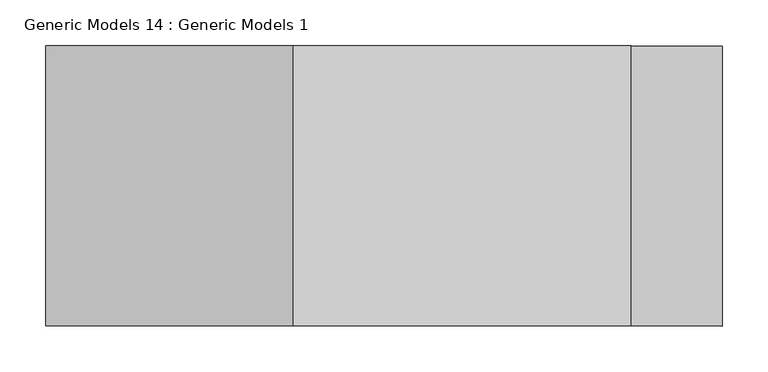
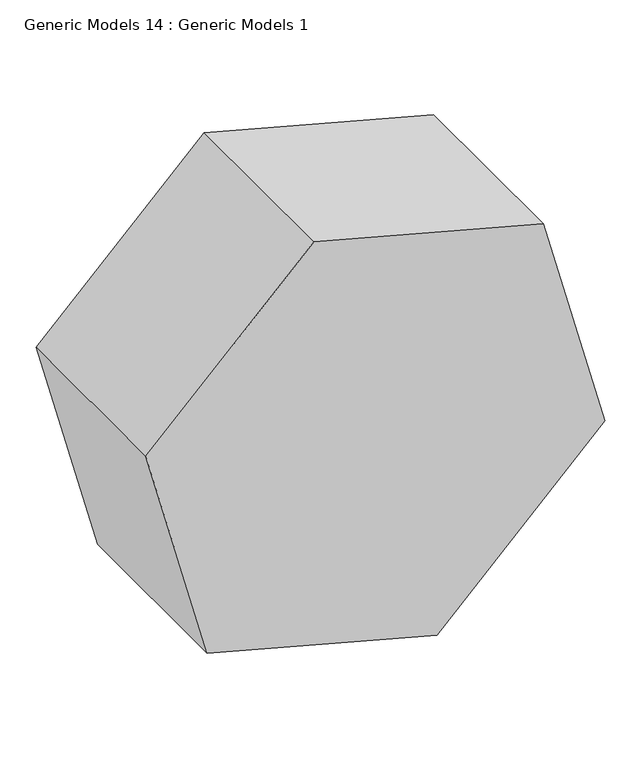
"""IFC4 building model written with IfcOpenShell, lengths in millimetres: proxy geometry, Generic Models 14 : Generic Models 1."""

from ifc_helpers import new_model, si_unit, frame, origin, place, context, project, spatial, polyline, outline, extrude, source, transform, mapped, element, save


def generic_models_14_generic_models_1_1a1bfa67(model_context):
    return source(origin(), model_context, "Body", "SweptSolid", [
        extrude(outline(polyline([(904.7566299, 5164.2198357), (1003.366686, 4796.2020959), (733.9590024, 4526.7944123), (365.9412626, 4625.4044685), (267.3312064, 4993.4222083), (536.73889, 5262.8298919), (904.7566299, 5164.2198357)])), frame((0.0, -9086.6225464, 0.0), z_axis=(0.0, 1.0, 0.0), x_axis=(0.0, 0.0, 1.0)), (0.0, 0.0, 1.0), 304.8),
    ])


if __name__ == "__main__":
    model = new_model("IFC4")
    model_context = context("Model", 3, world=origin())
    ifc_project = project(units=[si_unit("LENGTHUNIT", "METRE", prefix="MILLI")], contexts=[model_context])
    site = spatial("IfcSite", under=ifc_project)
    building = spatial("IfcBuilding", under=site)
    placement = place(None, origin())
    generic_models_14_generic_models_1_shape = generic_models_14_generic_models_1_1a1bfa67(model_context)
    element("IfcBuildingElementProxy", 1, Name="Generic Models 14 : Generic Models 1", ObjectType="Generic Models 14 : Generic Models 1", at=placement, inside=building, context=model_context, shape_type="MappedRepresentation", body=[
        mapped(generic_models_14_generic_models_1_shape, transform((0.0, 0.0, 0.0), x_axis=(1.0, 0.0, 0.0), y_axis=(0.0, 1.0, 0.0), z_axis=(0.0, 0.0, 1.0))),
    ])
    save(model, "model.ifc")

# Revit data of these elements
# Element 1 (IfcBuildingElementProxy, "Generic Models 14 : Generic Models 1")
#   Materials on its faces: "Brick, Common"
# Materials
#   "Brick, Common": class "Masonry", colour RGB 170 98 104, transparency 0, Description = "Common brick", Cost = 0
